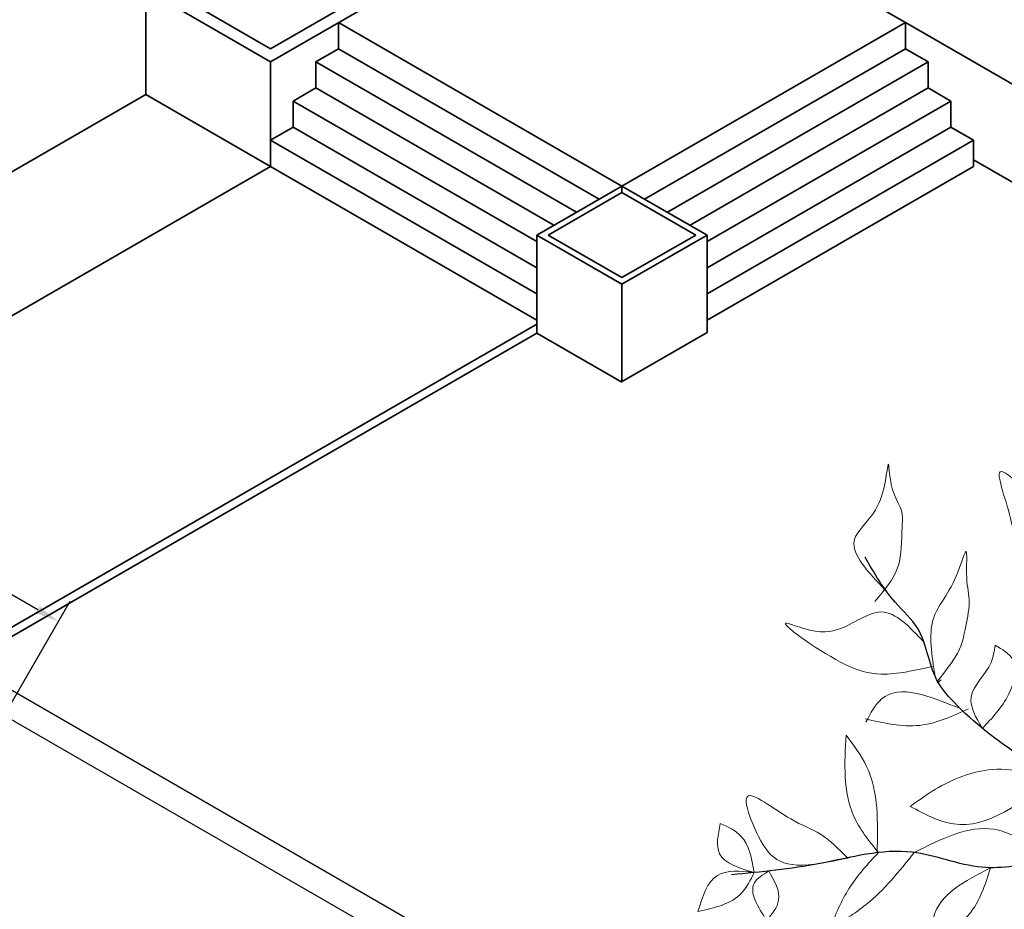
# Model space of a CAD drawing. Units: metres. Extents: x 12735 to 25554, y 20954 to 41989.
# Tile 4 of 15: x 12748.612 to 12756.135, y 20963.527 to 20970.327. Entities that reach past the tile are written whole.
import ezdxf

# ---------------------------------------------------------------- set-up
doc = ezdxf.new("R2010")
doc.units = ezdxf.units.M
doc.layers.get('Defpoints').update_dxf_attribs({"lineweight": 13})
for name, color, linetype, lineweight in [('A-ANNO-DIMS', 2, 'Continuous', 18), ('A-ELEV', 7, 'Continuous', 35), ('C-SITE', 8, 'Continuous', 25), ('TREES', 72, 'Continuous', 18)]:
    doc.layers.add(name, color=color, linetype=linetype, lineweight=lineweight)
doc.layers.add('STEM', color=32, linetype='Continuous')
doc.styles.get("Standard").update_dxf_attribs({"font": 'arial.ttf'})
doc.dimstyles.get("Standard").update_dxf_attribs({"dimtxt": 0.18, "dimasz": 0.18, "dimexe": 0.18, "dimexo": 0.0625, "dimgap": 0.09, "dimtad": 0, "dimtih": 1, "dimtoh": 1, "dimdec": 4, "dimzin": 0, "dimdsep": 46, "dimtxsty": 'Standard', "dimcen": 0.09, "dimadec": 0, "dimazin": 0, "dimtfac": 1, "dimtdec": 4, "dimtofl": 0, "dimtmove": 0, "dimatfit": 3, "dimfxl": 1, "dimtolj": 1, "dimtzin": 0, "dimarcsym": 0})

# ---------------------------------------------------------------- blocks, each defined once
blk = doc.blocks.new('TREES')
at = {"layer": 'STEM'}
for points, knots in [([(12743.7281, 20972.2176), (12743.6297, 20972.3723), (12743.3829, 20972.7603), (12742.7533, 20973.0696), (12742.2913, 20973.4192), (12741.9843, 20973.7592), (12741.9588, 20974.098), (12741.6755, 20974.3463), (12741.5627, 20974.5433), (12741.4939, 20974.6635)], [0, 0, 0, 0, 0.542161, 1.359078, 2.03444, 2.290187, 2.703676, 2.968549, 3.382864, 3.382864, 3.382864, 3.382864]), ([(12743.5969, 20972.4179), (12743.5329, 20972.4098), (12743.2921, 20972.3792), (12742.8892, 20972.3514), (12742.3639, 20972.2407), (12741.8027, 20972.4888), (12741.1572, 20972.3019), (12740.6984, 20972.2581), (12740.4736, 20972.2366)], [0, 0, 0, 0, 0.193148, 0.727923, 1.218416, 1.762371, 2.471743, 3.152626, 3.152626, 3.152626, 3.152626])]:
    blk.add_open_spline(points, degree=3, knots=knots, dxfattribs=at)
at = {"layer": 'TREES'}
for points, knots in [([(12741.6479, 20974.4113), (12741.5185, 20974.5473), (12741.2805, 20974.7977), (12741.6416, 20974.9951), (12741.6725, 20975.5108), (12741.6838, 20975.1491), (12741.7874, 20975.0327), (12741.7683, 20974.8245), (12741.781, 20974.5754), (12741.641, 20974.411), (12741.5686, 20974.3259)], [0, 0, 0, 0, 0.446457, 0.821839, 1.096823, 1.294203, 1.491123, 1.594729, 1.894892, 2.216107, 2.216107, 2.216107, 2.216107]), ([(12743.0703, 20974.7331), (12742.9798, 20974.8632), (12742.8479, 20975.0529), (12742.4329, 20975.446), (12742.6489, 20974.9152), (12742.6511, 20974.5734), (12742.9614, 20974.5759), (12743.0338, 20974.6779), (12743.0707, 20974.7298)], [0, 0, 0, 0, 0.54832, 0.799685, 1.166614, 1.565159, 1.742127, 1.925713, 1.925713, 1.925713, 1.925713]), ([(12742.0285, 20973.754), (12742.0027, 20973.9122), (12741.953, 20974.2176), (12742.1736, 20974.4138), (12742.2826, 20974.8097), (12742.2579, 20974.4803), (12742.3045, 20974.3234), (12742.2464, 20974.0686), (12742.2274, 20973.9317), (12742.0061, 20973.671), (12742.0659, 20973.7201), (12742.0748, 20973.7273)], [0, 0, 0, 0, 0.436736, 0.842969, 1.012738, 1.21393, 1.403734, 1.613178, 1.897283, 2.067562, 2.097274, 2.097274, 2.097274, 2.097274]), ([(12741.9427, 20974.0162), (12741.8348, 20974.1297), (12741.5945, 20974.3824), (12741.2715, 20973.9914), (12740.6869, 20974.2702), (12741.289, 20973.8358), (12741.6296, 20973.7415), (12741.8783, 20973.7991), (12742.0162, 20973.8311)], [0, 0, 0, 0, 0.397812, 0.88569, 1.156328, 1.66735, 1.991498, 2.394837, 2.394837, 2.394837, 2.394837]), ([(12742.3889, 20973.3561), (12742.3408, 20973.4372), (12742.2339, 20973.6174), (12742.4583, 20973.7994), (12742.4799, 20973.946), (12742.4865, 20973.9906)], [0, 0, 0, 0, 0.251735, 0.5591808, 0.6938707, 0.6938707, 0.6938707, 0.6938707]), ([(12742.4865, 20973.9906), (12742.5416, 20973.9591), (12742.6799, 20973.8802), (12742.5982, 20973.5723), (12742.4638, 20973.4334), (12742.3889, 20973.3561)], [0, 0, 0, 0, 0.1746142, 0.4385715, 0.7703441, 0.7703441, 0.7703441, 0.7703441]), ([(12742.2212, 20973.5061), (12741.9886, 20973.6018), (12741.6739, 20973.7313), (12741.5357, 20973.4714), (12741.4997, 20973.4036)], [0, 0, 0, 0, 0.6060397, 0.8197481, 0.8197481, 0.8197481, 0.8197481]), ([(12741.4934, 20973.4289), (12741.634, 20973.3961), (12741.9065, 20973.3326), (12742.1603, 20973.4486), (12742.2832, 20973.5046)], [0, 0, 0, 0, 0.420024, 0.8136231, 0.8136231, 0.8136231, 0.8136231]), ([(12741.5953, 20972.4061), (12741.5227, 20972.4964), (12741.3176, 20972.752), (12741.336, 20973.0874), (12741.348, 20973.3043)], [0, 0, 0, 0, 0.3390919, 0.9589007, 0.9589007, 0.9589007, 0.9589007]), ([(12741.348, 20973.3043), (12741.4064, 20973.2266), (12741.6002, 20972.9687), (12741.5913, 20972.6368), (12741.585, 20972.4049)], [0, 0, 0, 0, 0.2865181, 0.9509807, 0.9509807, 0.9509807, 0.9509807]), ([(12742.9828, 20972.9608), (12742.7991, 20973.0095), (12742.4631, 20973.0985), (12742.0708, 20972.9279), (12741.8932, 20972.7984), (12741.8387, 20972.7587)], [0, 0, 0, 0, 0.553894, 1.01265, 1.215779, 1.215779, 1.215779, 1.215779]), ([(12741.8387, 20972.7587), (12741.9489, 20972.7001), (12742.3229, 20972.5013), (12742.6839, 20972.7862), (12742.9385, 20972.9872)], [0, 0, 0, 0, 0.355589, 1.206871, 1.206871, 1.206871, 1.206871]), ([(12741.3584, 20972.3658), (12741.2913, 20972.4335), (12741.1619, 20972.5642), (12740.9085, 20972.6456), (12740.4916, 20972.9889), (12740.7191, 20972.3814), (12740.9045, 20972.2526), (12741.4371, 20972.382), (12741.3614, 20972.3664), (12741.3584, 20972.3658)], [0, 0, 0, 0, 0.274554, 0.529523, 0.902439, 1.220606, 1.740632, 1.953969, 1.962894, 1.962894, 1.962894, 1.962894]), ([(12740.6453, 20972.2539), (12740.5318, 20972.2869), (12740.3304, 20972.3454), (12740.37, 20972.5432), (12740.3873, 20972.6295)], [0, 0, 0, 0, 0.300298, 0.5327787, 0.5327787, 0.5327787, 0.5327787]), ([(12740.3873, 20972.6295), (12740.4457, 20972.6019), (12740.5975, 20972.5302), (12740.6271, 20972.3592), (12740.6453, 20972.2539)], [0, 0, 0, 0, 0.1847401, 0.4807235, 0.4807235, 0.4807235, 0.4807235]), ([(12742.9156, 20972.3429), (12742.7721, 20972.4516), (12742.4478, 20972.6972), (12742.0764, 20972.5107), (12741.8694, 20972.4068)], [0, 0, 0, 0, 0.501704, 1.133573, 1.133573, 1.133573, 1.133573]), ([(12741.2232, 20971.8233), (12741.3191, 20971.8812), (12741.5708, 20972.0332), (12741.7553, 20972.264), (12741.8694, 20972.4068)], [0, 0, 0, 0, 0.3340001, 0.876507, 0.876507, 0.876507, 0.876507]), ([(12741.5953, 20972.4061), (12741.515, 20972.319), (12741.3563, 20972.1468), (12741.2672, 20971.9303), (12741.2232, 20971.8233)], [0, 0, 0, 0, 0.3521388, 0.6963584, 0.6963584, 0.6963584, 0.6963584]), ([(12740.6453, 20972.2539), (12740.5405, 20972.2642), (12740.3185, 20972.2859), (12740.2516, 20972.0696), (12740.2163, 20971.9555)], [0, 0, 0, 0, 0.2808571, 0.5946199, 0.5946199, 0.5946199, 0.5946199]), ([(12740.2163, 20971.9555), (12740.3438, 20971.9838), (12740.536, 20972.0264), (12740.6178, 20972.1967), (12740.6453, 20972.2539)], [0, 0, 0, 0, 0.3624795, 0.5464116, 0.5464116, 0.5464116, 0.5464116]), ([(12740.7568, 20972.2652), (12740.7124, 20972.2374), (12740.5731, 20972.1499), (12740.6732, 20971.9932), (12740.7414, 20971.8865)], [0, 0, 0, 0, 0.1417373, 0.4445248, 0.4445248, 0.4445248, 0.4445248]), ([(12740.7414, 20971.8865), (12740.7826, 20971.9371), (12740.878, 20972.054), (12740.8007, 20972.1887), (12740.7568, 20972.2652)], [0, 0, 0, 0, 0.1798963, 0.4162104, 0.4162104, 0.4162104, 0.4162104]), ([(12742.4525, 20972.2905), (12742.2567, 20972.189), (12741.9991, 20972.0556), (12742.0012, 20971.792), (12742.0017, 20971.7289)], [0, 0, 0, 0, 0.5792647, 0.7616052, 0.7616052, 0.7616052, 0.7616052]), ([(12742.0017, 20971.7289), (12742.1084, 20971.7885), (12742.3333, 20971.9141), (12742.4115, 20972.1608), (12742.4525, 20972.2905)], [0, 0, 0, 0, 0.3533474, 0.7448355, 0.7448355, 0.7448355, 0.7448355])]:
    blk.add_open_spline(points, degree=3, knots=knots, dxfattribs=at)
blk = doc.blocks.new('*D9')
at = {"layer": 'A-ANNO-DIMS', "color": 0, "lineweight": -2, "transparency": 16777216}
for p, q in [((12781.0041, 20970.8701), (12781.0041, 20953.8934)), ((12737.8426, 20966.671), (12737.8426, 20953.8934)), ((12738.0226, 20954.0734), (12759.0261, 20954.0734)), ((12780.8241, 20954.0734), (12759.8206, 20954.0734))]:
    blk.add_line(p, q, dxfattribs=at)
at = {"layer": 'A-ANNO-DIMS', "color": 0, "transparency": 16777216}
for points in [[(12738.0226, 20954.1034), (12738.0226, 20954.0434), (12737.8426, 20954.0734)], [(12780.8241, 20954.1034), (12780.8241, 20954.0434), (12781.0041, 20954.0734)]]:
    blk.add_solid(points, dxfattribs=at)
at = {"layer": 'Defpoints', "color": 0, "transparency": 16777216}
for p in [(12781.0041, 20970.9326), (12737.8426, 20966.7335), (12781.0041, 20954.0734)]:
    blk.add_point(p, dxfattribs=at)
at = {"layer": 'A-ANNO-DIMS', "color": 0, "transparency": 16777216, "insert": (12759.4234, 20954.0734), "char_height": 0.18, "attachment_point": 5}
blk.add_mtext('\\A1;43.16', dxfattribs=at)
blk = doc.blocks.new('*D10')
at = {"layer": 'A-ANNO-DIMS', "color": 0, "lineweight": -2, "transparency": 16777216}
for p, q in [((12766.6445, 20994.8247), (12783.4841, 20994.8247)), ((12783.3041, 20994.6447), (12783.3041, 20975.781)), ((12783.3041, 20956.5534), (12783.3041, 20975.4171)), ((12755.8494, 20956.3734), (12783.4841, 20956.3734))]:
    blk.add_line(p, q, dxfattribs=at)
at = {"layer": 'A-ANNO-DIMS', "color": 0, "transparency": 16777216}
for points in [[(12783.2741, 20994.6447), (12783.3341, 20994.6447), (12783.3041, 20994.8247)], [(12783.2741, 20956.5534), (12783.3341, 20956.5534), (12783.3041, 20956.3734)]]:
    blk.add_solid(points, dxfattribs=at)
at = {"layer": 'Defpoints', "color": 0, "transparency": 16777216}
for p in [(12766.582, 20994.8247), (12783.3041, 20994.8247), (12755.7869, 20956.3734)]:
    blk.add_point(p, dxfattribs=at)
at = {"layer": 'A-ANNO-DIMS', "color": 0, "transparency": 16777216, "insert": (12783.3041, 20975.599), "char_height": 0.18, "attachment_point": 5}
blk.add_mtext('\\A1;38.45', dxfattribs=at)
blk = doc.blocks.new('*D11')
at = {"layer": 'A-ANNO-DIMS', "color": 0, "lineweight": -2, "transparency": 16777216}
for p, q in [((12737.8114, 20966.6794), (12736.6026, 20964.5857)), ((12736.8485, 20964.6516), (12745.3497, 20959.7435)), ((12754.481, 20954.4715), (12745.9798, 20959.3797)), ((12755.7556, 20956.3192), (12754.5469, 20954.2256))]:
    blk.add_line(p, q, dxfattribs=at)
at = {"layer": 'A-ANNO-DIMS', "color": 0, "transparency": 16777216}
for points in [[(12736.8635, 20964.6776), (12736.8335, 20964.6257), (12736.6926, 20964.7416)], [(12754.496, 20954.4975), (12754.466, 20954.4455), (12754.6369, 20954.3815)]]:
    blk.add_solid(points, dxfattribs=at)
at = {"layer": 'Defpoints', "color": 0, "transparency": 16777216}
for p in [(12737.8426, 20966.7335), (12736.6926, 20964.7416), (12755.7869, 20956.3734)]:
    blk.add_point(p, dxfattribs=at)
at = {"layer": 'A-ANNO-DIMS', "color": 0, "transparency": 16777216, "insert": (12745.6647, 20959.5616), "char_height": 0.18, "attachment_point": 5}
blk.add_mtext('\\A1;20.72', dxfattribs=at)
blk = doc.blocks.new('*D12')
at = {"layer": 'A-ANNO-DIMS', "color": 0, "lineweight": -2, "transparency": 16777216}
for p, q in [((12781.0354, 20970.8785), (12782.2441, 20968.7848)), ((12781.9983, 20968.8507), (12769.8606, 20961.843)), ((12757.0927, 20954.4715), (12769.2304, 20961.4792)), ((12755.8181, 20956.3192), (12757.0269, 20954.2256))]:
    blk.add_line(p, q, dxfattribs=at)
at = {"layer": 'A-ANNO-DIMS', "color": 0, "transparency": 16777216}
for points in [[(12781.9833, 20968.8767), (12782.0133, 20968.8247), (12782.1541, 20968.9407)], [(12757.0777, 20954.4975), (12757.1077, 20954.4455), (12756.9369, 20954.3815)]]:
    blk.add_solid(points, dxfattribs=at)
at = {"layer": 'Defpoints', "color": 0, "transparency": 16777216}
for p in [(12781.0041, 20970.9326), (12755.7869, 20956.3734), (12756.9369, 20954.3815)]:
    blk.add_point(p, dxfattribs=at)
at = {"layer": 'A-ANNO-DIMS', "color": 0, "transparency": 16777216, "insert": (12769.5455, 20961.6611), "char_height": 0.18, "attachment_point": 5}
blk.add_mtext('\\A1;29.12', dxfattribs=at)
blk = doc.blocks.new('*D24')
at = {"layer": 'A-ANNO-DIMS', "color": 0, "lineweight": -2, "transparency": 16777216}
for p, q in [((12744.4369, 20965.7244), (12745.6457, 20967.818)), ((12745.7116, 20967.5721), (12746.9163, 20966.8766)), ((12748.7514, 20965.8171), (12747.5467, 20966.5127)), ((12747.7885, 20963.7894), (12748.9973, 20965.883))]:
    blk.add_line(p, q, dxfattribs=at)
at = {"layer": 'A-ANNO-DIMS', "color": 0, "transparency": 16777216}
for points in [[(12745.7266, 20967.5981), (12745.6966, 20967.5462), (12745.5557, 20967.6621)], [(12748.7664, 20965.8431), (12748.7364, 20965.7911), (12748.9073, 20965.7271)]]:
    blk.add_solid(points, dxfattribs=at)
at = {"layer": 'Defpoints', "color": 0, "transparency": 16777216}
for p in [(12748.9073, 20965.7271), (12744.4057, 20965.6703), (12747.7573, 20963.7352)]:
    blk.add_point(p, dxfattribs=at)
at = {"layer": 'A-ANNO-DIMS', "color": 0, "transparency": 16777216, "insert": (12747.2315, 20966.6946), "char_height": 0.18, "attachment_point": 5}
blk.add_mtext('\\A1;3.87', dxfattribs=at)

msp = doc.modelspace()

# ---------------------------------------------------------------- linework, layer by layer
at = {"layer": 'A-ELEV'}
for p, q in [((12755.379, 20970.3057), (12752.2613, 20972.1057)), ((12750.5292, 20970.1057), (12753.1273, 20971.6057)), ((12750.5292, 20970.0057), (12753.2139, 20971.5557)), ((12750.5292, 20970.0057), (12749.5766, 20970.5557)), ((12749.5766, 20969.7557), (12749.5766, 20970.5557)), ((12750.5292, 20970.1057), (12749.7498, 20970.5557)), ((12753.2139, 20969.0557), (12751.0488, 20970.3057)), ((12751.0488, 20970.3057), (12751.0488, 20970.1057)), ((12755.379, 20970.3057), (12753.2139, 20969.0557)), ((12760.5269, 20967.3335), (12755.379, 20970.3057)), ((12755.379, 20970.3057), (12755.379, 20970.1057)), ((12751.0488, 20970.1057), (12750.8756, 20970.0057)), ((12751.0488, 20970.1057), (12753.0407, 20968.9557)), ((12755.379, 20970.1057), (12753.3871, 20968.9557)), ((12755.379, 20970.1057), (12755.5522, 20970.0057)), ((12750.5292, 20969.2057), (12750.5292, 20970.0057)), ((12750.8756, 20970.0057), (12752.8675, 20968.8557)), ((12750.8756, 20970.0057), (12750.8756, 20969.8057)), ((12755.5522, 20970.0057), (12753.5603, 20968.8557)), ((12755.5522, 20970.0057), (12755.5522, 20969.8057)), ((12749.5766, 20969.7557), (12744.6014, 20966.8833)), ((12750.5292, 20969.2057), (12749.5766, 20969.7557)), ((12750.8756, 20969.8057), (12750.7024, 20969.7057)), ((12750.8756, 20969.8057), (12752.6943, 20968.7557)), ((12755.5522, 20969.8057), (12753.7335, 20968.7557)), ((12755.5522, 20969.8057), (12753.7335, 20968.7557)), ((12755.5522, 20969.8057), (12755.7254, 20969.7057)), ((12750.7024, 20969.7057), (12752.5644, 20968.6307)), ((12750.7024, 20969.7057), (12750.7024, 20969.5057)), ((12755.7254, 20969.7057), (12753.8634, 20968.6307)), ((12755.7254, 20969.7057), (12755.7254, 20969.5057)), ((12750.7024, 20969.5057), (12750.5292, 20969.4057)), ((12750.7024, 20969.5057), (12752.5644, 20968.4307)), ((12755.7254, 20969.5057), (12753.8634, 20968.4307)), ((12755.7254, 20969.5057), (12753.8634, 20968.4307)), ((12755.7254, 20969.5057), (12755.8986, 20969.4057)), ((12750.5292, 20969.4057), (12752.5644, 20968.2307)), ((12750.5292, 20969.4057), (12750.5292, 20969.2057)), ((12755.8986, 20969.4057), (12753.8634, 20968.2307)), ((12755.8986, 20969.4057), (12755.8986, 20969.2057)), ((12760.5269, 20966.5835), (12755.8986, 20969.2557)), ((12744.4057, 20965.6703), (12750.5292, 20969.2057)), ((12750.5292, 20969.2057), (12752.5644, 20968.0307)), ((12755.8986, 20969.2057), (12753.8634, 20968.0307)), ((12755.8986, 20969.2057), (12753.8634, 20968.0307)), ((12753.2139, 20969.0557), (12752.5644, 20968.6807)), ((12753.2139, 20969.0057), (12752.651, 20968.6807)), ((12753.2139, 20969.0557), (12753.2139, 20969.0057)), ((12753.8634, 20968.6807), (12753.2139, 20969.0557)), ((12753.7768, 20968.6807), (12753.2139, 20969.0057)), ((12752.5644, 20967.9307), (12752.5644, 20968.6807)), ((12752.5644, 20968.6807), (12753.2139, 20968.3057)), ((12752.651, 20968.6807), (12753.2139, 20968.3557)), ((12753.2139, 20968.3057), (12753.8634, 20968.6807)), ((12753.2139, 20968.3557), (12753.7768, 20968.6807)), ((12753.8634, 20968.6807), (12753.8634, 20967.9357)), ((12753.2139, 20968.3057), (12753.2139, 20967.5557)), ((12752.5644, 20968.0001), (12748.1353, 20965.443)), ((12752.5644, 20967.9307), (12748.1954, 20965.4083)), ((12753.2139, 20967.5557), (12752.5644, 20967.9307)), ((12753.8634, 20967.9357), (12753.2096, 20967.5582))]:
    msp.add_line(p, q, dxfattribs=at)
at = {"layer": 'C-SITE'}
for p, q in [((12747.953, 20965.5482), (12757.9519, 20959.7754)), ((12747.7573, 20965.4352), (12757.9519, 20959.5494))]:
    msp.add_line(p, q, dxfattribs=at)

# ---------------------------------------------------------------- block references
at = {"layer": 'TREES'}
msp.add_blockref('TREES', (13.5777, -8.4449), dxfattribs=at)

# ---------------------------------------------------------------- dimensions: what is measured, and where the dimension line sits
at = {"layer": 'A-ANNO-DIMS'}
for base, p1, p2, angle, picture, middle in [((12783.3041, 20994.8247), (12755.7869, 20956.3734), (12766.582, 20994.8247), 90, '*D10', (12783.3041, 20975.599)), ((12756.9369, 20954.3815), (12781.0041, 20970.9326), (12755.7869, 20956.3734), 210, '*D12', (12769.5455, 20961.6611)), ((12748.9073, 20965.7271), (12744.4057, 20965.6703), (12747.7573, 20963.7352), 330, '*D24', (12747.2315, 20966.6946)), ((12736.6926, 20964.7416), (12755.7869, 20956.3734), (12737.8426, 20966.7335), 150, '*D11', (12745.6647, 20959.5616))]:
    dim = msp.add_linear_dim(base=base, p1=p1, p2=p2, angle=angle, dimstyle='Standard', override={"dimdec": 2, "dimlfac": 1, "dimrnd": 0, "dimzin": 0, "dimdsep": 46, "dimlunit": 2}, dxfattribs=at)
    dim.commit()
    dim.dimension.update_dxf_attribs({"geometry": picture, "text_midpoint": middle})
dim = msp.add_linear_dim(base=(12781.0041, 20954.0734), p1=(12737.8426, 20966.7335), p2=(12781.0041, 20970.9326), dimstyle='Standard', override={"dimdec": 2, "dimlfac": 1, "dimrnd": 0, "dimzin": 0, "dimdsep": 46, "dimlunit": 2}, dxfattribs=at)
dim.commit()
dim.dimension.update_dxf_attribs({"geometry": '*D9', "text_midpoint": (12759.4234, 20954.0734)})

doc.saveas('drawing.dxf')
